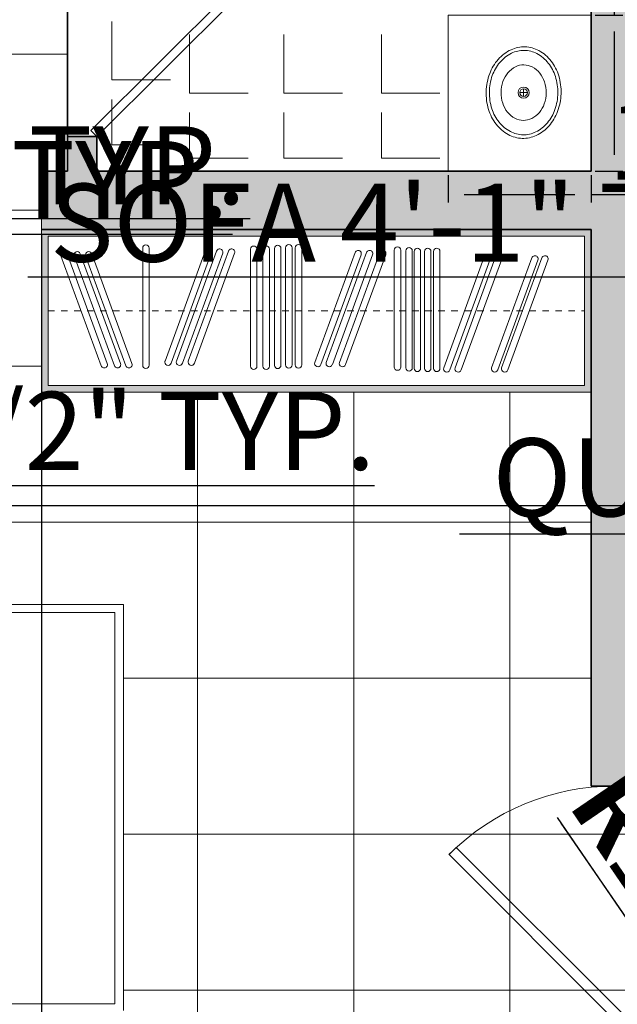
# Model space of a CAD drawing. Units: millimetres. Extents: x 542930 to 543750, y 628093 to 628738.
# Tile 4 of 14: x 543061 to 543153, y 628363 to 628514. Entities that reach past the tile are written whole.
import ezdxf

# ---------------------------------------------------------------- set-up
doc = ezdxf.new("R2010")
doc.units = ezdxf.units.MM
doc.linetypes.add('JIS_02_1.0', pattern=[2, 1, -1])
for name, color, linetype, lineweight in [('A-ANNO-DIMS', 2, 'Continuous', 18), ('A-FLOR-FIXT', 9, 'Continuous', 18), ('A-FURN', 8, 'Continuous', 18), ('A-FURN-MILL', 8, 'Continuous', 18), ('A-FURN-MILL-HIDN', 8, 'JIS_02_1.0', 13), ('A-FURN-PATT', 9, 'Continuous', 13), ('A-WALL', 7, 'Continuous', 35), ('DOORS', 30, 'Continuous', 18)]:
    doc.layers.add(name, color=color, linetype=linetype, lineweight=lineweight)
doc.layers.add('A-FLOR-PATT', color=241, linetype='Continuous', lineweight=13, true_color=0xf7abae)
doc.layers.add('A-WALL-PATT', color=251, linetype='Continuous', lineweight=13, true_color=0x636466)
doc.styles.get("Standard").update_dxf_attribs({"font": 'arial.ttf'})
doc.dimstyles.new('ISO-25', dxfattribs={"dimtxt": 12, "dimasz": 2.5, "dimexe": 1.25, "dimexo": 0.625, "dimtad": 1, "dimdec": 0, "dimlunit": 3, "dimtxsty": 'Standard', "dimcen": 2.5, "dimadec": 0, "dimazin": 0, "dimtfac": 1, "dimtdec": 0, "dimtmove": 0, "dimatfit": 3, "dimfxl": 1, "dimarcsym": 0})

# ---------------------------------------------------------------- blocks, each defined once
blk = doc.blocks.new('*U4')
for p, q in [((0, 0), (0, -6)), ((40, 0), (40, -6))]:
    blk.add_line(p, q)
blk.add_lwpolyline([(0, 0), (28.28, 28.28), (29.52, 27.05), (1.24, -1.24)], close=True)
blk.add_arc((0, 0), 40, 0, 45)
blk = doc.blocks.new('*U3')
for p, q in [((-40, 0), (-40, -6)), ((0, 0), (0, -6))]:
    blk.add_line(p, q)
blk.add_lwpolyline([(0, 0), (-28.28, 28.28), (-29.52, 27.05), (-1.24, -1.24)], close=True)
blk.add_arc((0, 0), 40, 135, 180)
blk = doc.blocks.new('Sink - Oval top')
for p, q in [((-1, 0), (1, 0)), ((0, 1), (0, -1))]:
    blk.add_line(p, q)
for points in [[(-12.23, 0.39, 0.117634), (-11.46, -3.36, 0.104469), (-8.88, -6.8, 0.090016), (-5.08, -9.07, 0.08192), (-0.32, -10.02, 0.08192), (4.49, -9.38, 0.090016), (8.42, -7.36, 0.104469), (11.22, -4.09, 0.117634), (12.23, -0.39, 0.117634), (11.46, 3.36, 0.104469), (8.88, 6.8, 0.090016), (5.08, 9.07, 0.08192), (0.32, 10.02, 0.08192), (-4.49, 9.38, 0.090016), (-8.42, 7.36, 0.104469), (-11.22, 4.09, 0.117634)], [(-11.29, 0.16, 0.118622), (-10.52, -3.25, 0.104678), (-8.07, -6.36, 0.089562), (-4.54, -8.37, 0.081185), (-0.13, -9.15, 0.081185), (4.3, -8.49, 0.089562), (7.89, -6.58, 0.104678), (10.42, -3.55, 0.118622), (11.29, -0.16, 0.118622), (10.52, 3.25, 0.104678), (8.07, 6.36, 0.089562), (4.54, 8.37, 0.081185), (0.13, 9.15, 0.081185), (-4.3, 8.49, 0.089562), (-7.89, 6.58, 0.104678), (-10.42, 3.55, 0.118622)], [(-7.42, 0.08, 0.118283), (-6.91, -2.17, 0.104607), (-5.29, -4.21, 0.089718), (-2.97, -5.53, 0.081436), (-0.07, -6.04, 0.081436), (2.84, -5.59, 0.089718), (5.2, -4.33, 0.104607), (6.86, -2.32, 0.118283), (7.42, -0.08, 0.118283), (6.91, 2.17, 0.104607), (5.29, 4.21, 0.089718), (2.97, 5.53, 0.081436), (0.07, 6.04, 0.081436), (-2.84, 5.59, 0.089718), (-5.2, 4.33, 0.104607), (-6.86, 2.32, 0.118283)]]:
    blk.add_lwpolyline(points, format="xyb", close=True)
for radius in [1.5, 1]:
    blk.add_circle((0, 0), radius)
blk = doc.blocks.new('Bed - Queen')
for p, q in [((0, -80.00003), (0, 0)), ((0, 0), (59.99999, 0)), ((59.99999, 0), (59.99999, -80.00003)), ((7.99999, -1.2), (28.79998, -1.2)), ((7.99999, -14.4), (7.99999, -1.2)), ((28.79998, -1.2), (28.79998, -14.4)), ((31.19999, -1.2), (51.99999, -1.2)), ((31.19999, -14.4), (31.19999, -1.2)), ((51.99999, -1.2), (51.99999, -16.4)), ((0, -14.4), (44.8, -14.4)), ((59.99999, -29.6), (44.8, -14.4)), ((44.8, -14.4), (44.8, -29.6)), ((51.99999, -16.4), (46.79936, -16.4)), ((44.8, -16.8), (0, -16.8)), ((44.8, -29.6), (59.99999, -29.6)), ((59.99999, -80.00003), (0, -80.00003))]:
    blk.add_line(p, q)
blk = doc.blocks.new('WARDROBE-BED-RAIL')
for p, q in [((0, 23), (0, 0)), ((0, 23), (82.5, 23)), ((82.5, 0), (82.5, 23)), ((8.16, 3.05), (1.98, 19.95)), ((9.1, 3.39), (2.92, 20.3)), ((10.2, 3.05), (4.02, 19.95)), ((11.14, 3.39), (4.96, 20.3)), ((11.95, 3.05), (5.77, 19.95)), ((12.89, 3.39), (6.71, 20.3)), ((14.55, 3.16), (14.55, 21.16)), ((15.55, 3.16), (15.55, 21.16)), ((17.99, 3.79), (24.17, 20.7)), ((18.92, 3.45), (25.1, 20.36)), ((19.74, 3.79), (25.92, 20.7)), ((20.68, 3.45), (26.86, 20.36)), ((21.57, 3.79), (27.75, 20.7)), ((22.51, 3.45), (28.69, 20.36)), ((31.12, 2.98), (31.12, 20.98)), ((32.12, 2.98), (32.12, 20.98)), ((33.04, 2.98), (33.04, 20.98)), ((34.04, 2.98), (34.04, 20.98)), ((34.81, 3.12), (34.81, 21.12)), ((35.81, 3.12), (35.81, 21.12)), ((36.51, 3.19), (36.51, 21.19)), ((37.51, 3.19), (37.51, 21.19)), ((38, 3.19), (38, 21.19)), ((39, 3.19), (39, 21.19)), ((41.02, 3.57), (47.2, 20.48)), ((41.96, 3.23), (48.14, 20.14)), ((42.77, 3.57), (48.95, 20.48)), ((43.71, 3.23), (49.89, 20.14)), ((44.81, 3.57), (50.99, 20.48)), ((45.75, 3.23), (51.93, 20.14)), ((53.23, 2.86), (53.23, 20.86)), ((54.23, 2.86), (54.23, 20.86)), ((55, 2.73), (55, 20.73)), ((56, 2.73), (56, 20.73)), ((56.28, 2.66), (56.28, 20.66)), ((57.28, 2.66), (57.28, 20.66)), ((57.87, 2.66), (57.87, 20.66)), ((58.87, 2.66), (58.87, 20.66)), ((59.26, 2.66), (59.26, 20.66)), ((60.26, 2.66), (60.26, 20.66)), ((60.83, 2.75), (67.01, 19.66)), ((61.77, 2.41), (67.95, 19.31)), ((62.58, 2.75), (68.76, 19.66)), ((63.52, 2.41), (69.7, 19.31)), ((68.19, 2.75), (74.37, 19.66)), ((69.13, 2.41), (75.31, 19.31)), ((69.74, 2.75), (75.92, 19.66)), ((70.68, 2.41), (76.86, 19.31)), ((0, 0), (82.5, 0))]:
    blk.add_line(p, q)
for centre, start, end in [((15.05, 21.16), 0, 180), ((31.62, 20.98), 0, 180), ((33.54, 20.98), 0, 180), ((35.31, 21.12), 0, 180), ((37.01, 21.19), 0, 180), ((38.5, 21.19), 0, 180), ((53.73, 20.86), 0, 180), ((55.5, 20.73), 0, 180), ((2.45, 20.12), 20.081, 200.081), ((4.49, 20.12), 20.081, 200.081), ((6.24, 20.12), 20.081, 200.081), ((24.63, 20.53), 339.919, 159.919), ((26.39, 20.53), 339.919, 159.919), ((28.22, 20.53), 339.919, 159.919), ((47.67, 20.31), 339.919, 159.919), ((49.42, 20.31), 339.919, 159.919), ((51.46, 20.31), 339.919, 159.919), ((56.78, 20.66), 0, 180), ((58.37, 20.66), 0, 180), ((59.76, 20.66), 0, 180), ((67.48, 19.49), 339.919, 159.919), ((69.23, 19.49), 339.919, 159.919), ((74.84, 19.49), 339.919, 159.919), ((76.39, 19.49), 339.919, 159.919), ((8.63, 3.22), 200.081, 20.081), ((10.67, 3.22), 200.081, 20.081), ((12.42, 3.22), 200.081, 20.081), ((15.05, 3.16), 180, 0), ((18.45, 3.62), 159.919, 339.919), ((20.21, 3.62), 159.919, 339.919), ((22.04, 3.62), 159.919, 339.919), ((35.31, 3.12), 180, 0), ((37.01, 3.19), 180, 0), ((38.5, 3.19), 180, 0), ((41.49, 3.4), 159.919, 339.919), ((43.24, 3.4), 159.919, 339.919), ((45.28, 3.4), 159.919, 339.919), ((31.62, 2.98), 180, 0), ((33.54, 2.98), 180, 0), ((53.73, 2.86), 180, 0), ((55.5, 2.73), 180, 0), ((56.78, 2.66), 180, 0), ((58.37, 2.66), 180, 0), ((59.76, 2.66), 180, 0), ((61.3, 2.58), 159.919, 339.919), ((63.05, 2.58), 159.919, 339.919), ((68.66, 2.58), 159.919, 339.919), ((70.21, 2.58), 159.919, 339.919)]:
    blk.add_arc(centre, 0.5, start, end)
blk = doc.blocks.new('LAVATORY-COUNTER')
for p, q in [((0, 0), (0, 24)), ((0, 24), (22, 24))]:
    blk.add_line(p, q)
blk = doc.blocks.new('*D32')
at = {"layer": 'A-ANNO-DIMS', "color": 0, "lineweight": -2, "transparency": 16777216}
for p, q in [((543011.12, 628481.15), (543008.62, 628481.15)), ((543013.62, 628478.92), (543013.62, 628482.4)), ((543013.62, 628481.15), (543014.62, 628481.15)), ((543014.62, 628478.92), (543014.62, 628482.4)), ((543017.12, 628481.15), (543094.01, 628481.15))]:
    blk.add_line(p, q, dxfattribs=at)
at = {"layer": 'A-ANNO-DIMS', "color": 0, "transparency": 16777216}
for points in [[(543011.12, 628481.56), (543011.12, 628480.73), (543013.62, 628481.15)], [(543017.12, 628481.56), (543017.12, 628480.73), (543014.62, 628481.15)]]:
    blk.add_solid(points, dxfattribs=at)
at = {"layer": 'Defpoints', "color": 0, "transparency": 16777216}
for p in [(543014.62, 628481.15), (543013.62, 628478.3), (543014.62, 628478.3)]:
    blk.add_point(p, dxfattribs=at)
at = {"layer": 'A-ANNO-DIMS', "color": 0, "transparency": 16777216, "insert": (543056.82, 628487.9), "char_height": 12, "attachment_point": 5}
blk.add_mtext('0\'-1" TYP.', dxfattribs=at)
blk = doc.blocks.new('*D33')
at = {"layer": 'A-ANNO-DIMS', "color": 0, "lineweight": -2, "transparency": 16777216}
for p, q in [((543189.7, 628481.25), (543189.7, 628473.25)), ((543238.84, 628481.25), (543238.84, 628473.25)), ((543189.7, 628474.5), (543062.56, 628474.5)), ((543236.34, 628474.5), (543192.2, 628474.5))]:
    blk.add_line(p, q, dxfattribs=at)
at = {"layer": 'A-ANNO-DIMS', "color": 0, "transparency": 16777216}
for points in [[(543192.2, 628474.92), (543192.2, 628474.09), (543189.7, 628474.5)], [(543236.34, 628474.92), (543236.34, 628474.09), (543238.84, 628474.5)]]:
    blk.add_solid(points, dxfattribs=at)
at = {"layer": 'Defpoints', "color": 0, "transparency": 16777216}
for p in [(543189.7, 628481.87), (543238.84, 628481.87), (543189.7, 628474.5)]:
    blk.add_point(p, dxfattribs=at)
at = {"layer": 'A-ANNO-DIMS', "color": 0, "transparency": 16777216, "insert": (543124.88, 628481.34), "char_height": 12, "attachment_point": 5}
blk.add_mtext('SOFA 4\'-1" TYP.', dxfattribs=at)
blk = doc.blocks.new('*D37')
at = {"layer": 'A-ANNO-DIMS', "color": 0, "lineweight": -2, "transparency": 16777216}
for p, q in [((543337.17, 628423.55), (543337.17, 628436.21)), ((543417.44, 628423.55), (543417.44, 628436.21)), ((543337.17, 628434.96), (543128.93, 628434.96)), ((543414.94, 628434.96), (543339.67, 628434.96))]:
    blk.add_line(p, q, dxfattribs=at)
at = {"layer": 'A-ANNO-DIMS', "color": 0, "transparency": 16777216}
for points in [[(543339.67, 628435.38), (543339.67, 628434.55), (543337.17, 628434.96)], [(543414.94, 628435.38), (543414.94, 628434.55), (543417.44, 628434.96)]]:
    blk.add_solid(points, dxfattribs=at)
at = {"layer": 'Defpoints', "color": 0, "transparency": 16777216}
for p in [(543337.17, 628434.96), (543337.17, 628422.92), (543417.44, 628422.92)]:
    blk.add_point(p, dxfattribs=at)
at = {"layer": 'A-ANNO-DIMS', "color": 0, "transparency": 16777216, "insert": (543231.8, 628442.16), "char_height": 12, "attachment_point": 5}
blk.add_mtext('QUEEN BED 6\'-8 1/2" TYP.', dxfattribs=at)
blk = doc.blocks.new('*D44')
at = {"layer": 'A-ANNO-DIMS', "color": 0, "lineweight": -2, "transparency": 16777216}
for p, q in [((542994.67, 628492.2), (542994.67, 628482.28)), ((543019.67, 628492.2), (543019.67, 628482.28)), ((542997.17, 628483.53), (543017.17, 628483.53)), ((543019.67, 628483.53), (543096.77, 628483.53))]:
    blk.add_line(p, q, dxfattribs=at)
at = {"layer": 'A-ANNO-DIMS', "color": 0, "transparency": 16777216}
for points in [[(542997.17, 628483.94), (542997.17, 628483.11), (542994.67, 628483.53)], [(543017.17, 628483.94), (543017.17, 628483.11), (543019.67, 628483.53)]]:
    blk.add_solid(points, dxfattribs=at)
at = {"layer": 'Defpoints', "color": 0, "transparency": 16777216}
for p in [(542994.67, 628492.83), (543019.67, 628492.83), (543019.67, 628483.53)]:
    blk.add_point(p, dxfattribs=at)
at = {"layer": 'A-ANNO-DIMS', "color": 0, "transparency": 16777216, "insert": (543059.47, 628490.18), "char_height": 12, "attachment_point": 5}
blk.add_mtext('2\'-1" TYP.', dxfattribs=at)
blk = doc.blocks.new('*D55')
at = {"layer": 'A-ANNO-DIMS', "color": 0, "lineweight": -2, "transparency": 16777216}
for p, q in [((543152.77, 628514.83), (543152.77, 628679.13)), ((543149.79, 628514.83), (543154.02, 628514.83)), ((543152.77, 628493.33), (543152.77, 628512.33)), ((543149.79, 628490.83), (543154.02, 628490.83))]:
    blk.add_line(p, q, dxfattribs=at)
at = {"layer": 'A-ANNO-DIMS', "color": 0, "transparency": 16777216}
for points in [[(543152.35, 628512.33), (543153.18, 628512.33), (543152.77, 628514.83)], [(543152.35, 628493.33), (543153.18, 628493.33), (543152.77, 628490.83)]]:
    blk.add_solid(points, dxfattribs=at)
at = {"layer": 'Defpoints', "color": 0, "transparency": 16777216}
for p in [(543149.17, 628514.83), (543152.77, 628514.83), (543149.17, 628490.83)]:
    blk.add_point(p, dxfattribs=at)
at = {"layer": 'A-ANNO-DIMS', "color": 0, "transparency": 16777216, "insert": (543145.93, 628598.23), "char_height": 12, "attachment_point": 5, "rotation": 90}
blk.add_mtext('COUNTER 2\'-0" TYP.', dxfattribs=at)
blk = doc.blocks.new('*D56')
at = {"layer": 'A-ANNO-DIMS', "color": 0, "lineweight": -2, "transparency": 16777216}
for p, q in [((543127.17, 628490.2), (543127.17, 628485.98)), ((543149.17, 628490.2), (543149.17, 628485.98)), ((543129.67, 628487.23), (543146.67, 628487.23)), ((543149.17, 628487.23), (543234.26, 628487.23))]:
    blk.add_line(p, q, dxfattribs=at)
at = {"layer": 'A-ANNO-DIMS', "color": 0, "transparency": 16777216}
for points in [[(543129.67, 628487.64), (543129.67, 628486.81), (543127.17, 628487.23)], [(543146.67, 628487.64), (543146.67, 628486.81), (543149.17, 628487.23)]]:
    blk.add_solid(points, dxfattribs=at)
at = {"layer": 'Defpoints', "color": 0, "transparency": 16777216}
for p in [(543127.17, 628490.83), (543149.17, 628490.83), (543149.17, 628487.23)]:
    blk.add_point(p, dxfattribs=at)
at = {"layer": 'A-ANNO-DIMS', "color": 0, "transparency": 16777216, "insert": (543192.96, 628493.98), "char_height": 12, "attachment_point": 5}
blk.add_mtext('1\'-10" TYP.', dxfattribs=at)
blk = doc.blocks.new('*D60')
at = {"layer": 'A-ANNO-DIMS', "color": 0, "lineweight": -2, "transparency": 16777216}
for p, q in [((542992.67, 628439.52), (542992.67, 628443.74)), ((543012.12, 628439.52), (543012.12, 628443.74)), ((542995.17, 628442.49), (543009.62, 628442.49)), ((543012.12, 628442.49), (543115.85, 628442.49))]:
    blk.add_line(p, q, dxfattribs=at)
at = {"layer": 'A-ANNO-DIMS', "color": 0, "transparency": 16777216}
for points in [[(542995.17, 628442.91), (542995.17, 628442.08), (542992.67, 628442.49)], [(543009.62, 628442.91), (543009.62, 628442.08), (543012.12, 628442.49)]]:
    blk.add_solid(points, dxfattribs=at)
at = {"layer": 'Defpoints', "color": 0, "transparency": 16777216}
for p in [(543012.12, 628442.49), (542992.67, 628438.89), (543012.12, 628438.89)]:
    blk.add_point(p, dxfattribs=at)
at = {"layer": 'A-ANNO-DIMS', "color": 0, "transparency": 16777216, "insert": (543065.24, 628449.32), "char_height": 12, "attachment_point": 5}
blk.add_mtext('1\'-7 1/2" TYP.', dxfattribs=at)
blk = doc.blocks.new('*D75')
at = {"layer": 'A-ANNO-DIMS', "color": 0, "lineweight": -2, "transparency": 16777216}
for p, q in [((543324.54, 628439.36), (542953.72, 628439.36)), ((542954.97, 628352.33), (542954.97, 628436.86)), ((543324.54, 628349.83), (542953.72, 628349.83))]:
    blk.add_line(p, q, dxfattribs=at)
at = {"layer": 'A-ANNO-DIMS', "color": 0, "transparency": 16777216}
for points in [[(542954.55, 628436.86), (542955.38, 628436.86), (542954.97, 628439.36)], [(542954.55, 628352.33), (542955.38, 628352.33), (542954.97, 628349.83)]]:
    blk.add_solid(points, dxfattribs=at)
at = {"layer": 'Defpoints', "color": 0, "transparency": 16777216}
for p in [(542954.97, 628439.36), (543325.17, 628439.36), (543325.17, 628349.83)]:
    blk.add_point(p, dxfattribs=at)
at = {"layer": 'A-ANNO-DIMS', "color": 0, "transparency": 16777216, "insert": (542948.14, 628394.6), "char_height": 12, "attachment_point": 5, "rotation": 90}
blk.add_mtext('7\'-5 1/2"', dxfattribs=at)
blk = doc.blocks.new('*D85')
at = {"layer": 'A-ANNO-DIMS', "color": 0, "lineweight": -2, "transparency": 16777216}
for p, q in [((543028.62, 628481.2), (543028.62, 628103.84)), ((543064.67, 628481.2), (543064.67, 628103.84)), ((543031.12, 628105.09), (543062.17, 628105.09))]:
    blk.add_line(p, q, dxfattribs=at)
at = {"layer": 'A-ANNO-DIMS', "color": 0, "transparency": 16777216}
for points in [[(543031.12, 628105.5), (543031.12, 628104.67), (543028.62, 628105.09)], [(543062.17, 628105.5), (543062.17, 628104.67), (543064.67, 628105.09)]]:
    blk.add_solid(points, dxfattribs=at)
at = {"layer": 'Defpoints', "color": 0, "transparency": 16777216}
for p in [(543028.62, 628481.83), (543064.67, 628481.83), (543064.67, 628105.09)]:
    blk.add_point(p, dxfattribs=at)
at = {"layer": 'A-ANNO-DIMS', "color": 0, "transparency": 16777216, "insert": (543046.65, 628111.84), "char_height": 12, "attachment_point": 5}
blk.add_mtext('3\'-0"', dxfattribs=at)
blk = doc.blocks.new('*D94')
at = {"layer": 'A-ANNO-DIMS', "color": 0, "lineweight": -2, "transparency": 16777216}
for p, q in [((543143.96, 628391.37), (543186.37, 628329.39)), ((543198.34, 628311.9), (543187.78, 628327.33))]:
    blk.add_line(p, q, dxfattribs=at)
at = {"layer": 'A-ANNO-DIMS', "color": 0, "transparency": 16777216}
blk.add_solid([(543186.71, 628329.63), (543186.02, 628329.15), (543187.78, 628327.33)], dxfattribs=at)
at = {"layer": 'Defpoints', "color": 0, "transparency": 16777216}
for p in [(543187.78, 628327.33), (543198.34, 628311.9)]:
    blk.add_point(p, dxfattribs=at)
at = {"layer": 'A-ANNO-DIMS', "color": 0, "transparency": 16777216, "insert": (543170.1, 628365.27), "char_height": 12, "attachment_point": 5, "rotation": 304.3793}
blk.add_mtext('R1\'-6 1/2"', dxfattribs=at)
blk = doc.blocks.new('*D95')
at = {"layer": 'A-ANNO-DIMS', "color": 0, "lineweight": -2, "transparency": 16777216}
for p, q in [((543144.53, 628390.54), (543186.93, 628328.57)), ((543198.34, 628311.9), (543188.34, 628326.5))]:
    blk.add_line(p, q, dxfattribs=at)
at = {"layer": 'A-ANNO-DIMS', "color": 0, "transparency": 16777216}
blk.add_solid([(543187.28, 628328.8), (543186.59, 628328.33), (543188.34, 628326.5)], dxfattribs=at)
at = {"layer": 'Defpoints', "color": 0, "transparency": 16777216}
for p in [(543188.34, 628326.5), (543198.34, 628311.9)]:
    blk.add_point(p, dxfattribs=at)
at = {"layer": 'A-ANNO-DIMS', "color": 0, "transparency": 16777216, "insert": (543170.66, 628364.44), "char_height": 12, "attachment_point": 5, "rotation": 304.3778}
blk.add_mtext('R1\'-5 1/2"', dxfattribs=at)

msp = doc.modelspace()

# ---------------------------------------------------------------- hatches: boundary and pattern name
at = {"layer": 'A-FURN-PATT'}
h = msp.add_hatch(color=256, dxfattribs=at)
h.dxf.hatch_style = 1
h.paths.add_polyline_path([(543149.17, 628481.83), (543064.67, 628481.83), (543064.67, 628456.83), (543149.17, 628456.83)])
h.paths.add_polyline_path([(543065.67, 628480.83), (543148.17, 628480.83), (543148.17, 628457.83), (543065.67, 628457.83)], flags=16)
h.paths.add_polyline_path([(543067.65, 628477.78, -1), (543068.59, 628478.12), (543071.8, 628469.33), (543072.77, 628469.33), (543069.68, 628477.78, -1), (543070.62, 628478.12), (543073.84, 628469.33), (543074.53, 628469.33), (543071.44, 628477.78, -1), (543072.38, 628478.12), (543075.59, 628469.33), (543080.22, 628469.33), (543080.22, 628478.99, -1), (543081.22, 628478.99), (543081.22, 628469.33), (543086.47, 628469.33), (543089.83, 628478.53, -1), (543090.77, 628478.18), (543087.53, 628469.33), (543088.22, 628469.33), (543091.59, 628478.53, -1), (543092.53, 628478.18), (543089.29, 628469.33), (543090.05, 628469.33), (543093.41, 628478.53, -1), (543094.35, 628478.18), (543091.11, 628469.33), (543096.79, 628469.33), (543096.79, 628478.81, -1), (543097.79, 628478.81), (543097.79, 628469.33), (543098.7, 628469.33), (543098.7, 628478.81, -1), (543099.7, 628478.81), (543099.7, 628469.33), (543100.48, 628469.33), (543100.48, 628478.95, -1), (543101.48, 628478.95), (543101.48, 628469.33), (543102.18, 628469.33), (543102.18, 628479.02, -1), (543103.18, 628479.02), (543103.18, 628469.33), (543103.67, 628469.33), (543103.67, 628479.02, -1), (543104.67, 628479.02), (543104.67, 628469.33), (543109.58, 628469.33), (543112.87, 628478.31, -1), (543113.81, 628477.96), (543110.65, 628469.33), (543111.34, 628469.33), (543114.62, 628478.31, -1), (543115.56, 628477.96), (543112.4, 628469.33), (543113.38, 628469.33), (543116.66, 628478.31, -1), (543117.6, 628477.96), (543114.44, 628469.33), (543118.89, 628469.33), (543118.89, 628478.68, -1), (543119.89, 628478.68), (543119.89, 628469.33), (543120.67, 628469.33), (543120.67, 628478.56, -1), (543121.67, 628478.56), (543121.67, 628469.33), (543121.95, 628469.33), (543121.95, 628478.49, -1), (543122.95, 628478.49), (543122.95, 628469.33), (543123.53, 628469.33), (543123.53, 628478.49, -1), (543124.53, 628478.49), (543124.53, 628469.33), (543124.93, 628469.33), (543124.93, 628478.49, -1), (543125.93, 628478.49), (543125.93, 628469.33), (543129.69, 628469.33), (543132.68, 628477.48, -1), (543133.61, 628477.14), (543130.76, 628469.33), (543131.45, 628469.33), (543134.43, 628477.48, -1), (543135.37, 628477.14), (543132.51, 628469.33), (543137.05, 628469.33), (543140.03, 628477.48, -1), (543140.97, 628477.14), (543138.12, 628469.33), (543138.6, 628469.33), (543141.59, 628477.48, -1), (543142.52, 628477.14), (543136.34, 628460.23, -1), (543135.41, 628460.58), (543138.6, 628469.33), (543138.12, 628469.33), (543134.79, 628460.23, -1), (543133.85, 628460.58), (543137.05, 628469.33), (543132.51, 628469.33), (543129.19, 628460.23, -1), (543128.25, 628460.58), (543131.45, 628469.33), (543130.76, 628469.33), (543127.43, 628460.23, -1), (543126.5, 628460.58), (543129.69, 628469.33), (543125.93, 628469.33), (543125.93, 628460.49, -1), (543124.93, 628460.49), (543124.93, 628469.33), (543124.53, 628469.33), (543124.53, 628460.49, -1), (543123.53, 628460.49), (543123.53, 628469.33), (543122.95, 628469.33), (543122.95, 628460.49, -1), (543121.95, 628460.49), (543121.95, 628469.33), (543121.67, 628469.33), (543121.67, 628460.56, -1), (543120.67, 628460.56), (543120.67, 628469.33), (543119.89, 628469.33), (543119.89, 628460.68, -1), (543118.89, 628460.68), (543118.89, 628469.33), (543114.44, 628469.33), (543111.42, 628461.06, -1), (543110.48, 628461.4), (543113.38, 628469.33), (543112.4, 628469.33), (543109.38, 628461.06, -1), (543108.44, 628461.4), (543111.34, 628469.33), (543110.65, 628469.33), (543107.63, 628461.06, -1), (543106.69, 628461.4), (543109.58, 628469.33), (543104.67, 628469.33), (543104.67, 628461.02, -1), (543103.67, 628461.02), (543103.67, 628469.33), (543103.18, 628469.33), (543103.18, 628461.02, -1), (543102.18, 628461.02), (543102.18, 628469.33), (543101.48, 628469.33), (543101.48, 628460.95, -1), (543100.48, 628460.95), (543100.48, 628469.33), (543099.7, 628469.33), (543099.7, 628460.81, -1), (543098.7, 628460.81), (543098.7, 628469.33), (543097.79, 628469.33), (543097.79, 628460.81, -1), (543096.79, 628460.81), (543096.79, 628469.33), (543091.11, 628469.33), (543088.17, 628461.28, -1), (543087.23, 628461.62), (543090.05, 628469.33), (543089.29, 628469.33), (543086.35, 628461.28, -1), (543085.41, 628461.62), (543088.22, 628469.33), (543087.53, 628469.33), (543084.59, 628461.28, -1), (543083.65, 628461.62), (543086.47, 628469.33), (543081.22, 628469.33), (543081.22, 628460.99, -1), (543080.22, 628460.99), (543080.22, 628469.33), (543075.59, 628469.33), (543078.56, 628461.22, -1), (543077.62, 628460.87), (543074.53, 628469.33), (543073.84, 628469.33), (543076.8, 628461.22, -1), (543075.86, 628460.87), (543072.77, 628469.33), (543071.8, 628469.33), (543074.77, 628461.22, -1), (543073.83, 628460.87)], flags=0)
at = {"layer": 'A-WALL-PATT'}
h = msp.add_hatch(color=256, dxfattribs=at)
h.dxf.hatch_style = 1
h.paths.add_polyline_path([(543158.17, 628580.83), (543211.67, 628580.83), (543211.67, 628589.83), (543137.07, 628589.83), (543137.07, 628580.83), (543149.17, 628580.83), (543149.17, 628490.83), (543073.17, 628490.83), (543073.17, 628496.14), (543068.67, 628496.14), (543068.67, 628490.83), (543064.67, 628490.83), (543064.67, 628481.83), (543149.17, 628481.83), (543149.17, 628396.23), (543158.17, 628396.23)])

# ---------------------------------------------------------------- linework, layer by layer
at = {"layer": 'A-FLOR-PATT'}
for p, q in [((543075.49, 628513.86), (543075.49, 628504.86)), ((543087.43, 628511.83), (543087.43, 628502.83)), ((543101.92, 628511.83), (543101.92, 628502.83)), ((543116.93, 628511.83), (543116.93, 628502.83)), ((543021.67, 628508.83), (543068.67, 628508.83)), ((543075.49, 628504.86), (543084.49, 628504.86)), ((543087.43, 628502.83), (543096.43, 628502.83)), ((543101.92, 628502.83), (543110.92, 628502.83)), ((543116.93, 628502.83), (543125.93, 628502.83)), ((543075.49, 628501.86), (543075.49, 628494.86)), ((543087.43, 628499.83), (543087.43, 628492.83)), ((543101.92, 628499.83), (543101.92, 628492.83)), ((543116.93, 628499.83), (543116.93, 628492.83)), ((543075.49, 628494.86), (543084.49, 628494.86)), ((543087.43, 628492.83), (543096.43, 628492.83)), ((543101.92, 628492.83), (543110.92, 628492.83)), ((543116.93, 628492.83), (543125.93, 628492.83)), ((543028.62, 628484.83), (543064.67, 628484.83)), ((543028.62, 628460.83), (543064.67, 628460.83)), ((543088.67, 628262.83), (543088.67, 628456.83)), ((543112.67, 628262.83), (543112.67, 628456.83)), ((543136.67, 628262.83), (543136.67, 628456.83)), ((543012.12, 628436.83), (543149.17, 628436.83)), ((543077.27, 628412.83), (543149.17, 628412.83)), ((543077.27, 628388.83), (543304.67, 628388.83)), ((543077.27, 628364.83), (543304.67, 628364.83))]:
    msp.add_line(p, q, dxfattribs=at)
at = {"layer": 'A-FURN'}
for p, q in [((543012.12, 628424.17), (543077.27, 628424.17)), ((543077.27, 628424.17), (543077.27, 628361.72))]:
    msp.add_line(p, q, dxfattribs=at)
at = {"layer": 'A-FURN-MILL'}
for p, q in [((543064.67, 628490.83), (543064.67, 628456.83)), ((543064.67, 628456.83), (543149.17, 628456.83))]:
    msp.add_line(p, q, dxfattribs=at)
at = {"layer": 'A-FURN-MILL-HIDN'}
msp.add_line((543065.67, 628469.33), (543148.17, 628469.33), dxfattribs=at)
at = {"layer": 'A-WALL'}
for p, q in [((543068.67, 628490.83), (543068.67, 628580.83)), ((543149.17, 628490.83), (543149.17, 628580.83)), ((543068.67, 628496.14), (543073.17, 628496.14)), ((543073.17, 628490.83), (543073.17, 628496.14)), ((543064.67, 628490.83), (543068.67, 628490.83)), ((543073.17, 628490.83), (543149.17, 628490.83)), ((543064.67, 628481.83), (543149.17, 628481.83)), ((543149.17, 628396.23), (543149.17, 628481.83)), ((543158.17, 628396.23), (543149.17, 628396.23))]:
    msp.add_line(p, q, dxfattribs=at)

# ---------------------------------------------------------------- block references
at = {"layer": 'A-FLOR-FIXT'}
msp.add_blockref('LAVATORY-COUNTER', (543127.17, 628490.83), dxfattribs=at)
at = {"layer": 'A-FLOR-FIXT', "xscale": 0.5752271451798996, "yscale": 0.5752271451798996, "zscale": 0.5752271451798996, "rotation": 270}
msp.add_blockref('Sink - Oval top', (543138.79, 628502.91), dxfattribs=at)
at = {"layer": 'A-FURN', "xscale": 1.003451310197957, "yscale": 1.003451310197957, "zscale": 1.003451310197957, "rotation": 90}
msp.add_blockref('Bed - Queen', (542995.67, 628362.72), dxfattribs=at)
at = {"layer": 'A-FURN-MILL'}
msp.add_blockref('WARDROBE-BED-RAIL', (543065.67, 628457.83), dxfattribs=at)
at = {"layer": 'DOORS'}
for name, p, xscale, yscale, zscale, rotation in [('*U3', (543073.17, 628496.14), 0.75, 0.75, 0.75, 270), ('*U4', (543152.77, 628360.23), 0.9000000000029102, 0.9000000000029102, 0.9000000000029102, 90)]:
    msp.add_blockref(name, p, dxfattribs=dict(at, xscale=xscale, yscale=yscale, zscale=zscale, rotation=rotation))

# ---------------------------------------------------------------- dimensions: what is measured, and where the dimension line sits
at = {"layer": 'A-ANNO-DIMS'}
for base, p1, p2, angle, text, picture, middle in [((543152.77, 628514.83), (543149.17, 628490.83), (543149.17, 628514.83), 90, 'COUNTER <> TYP.', '*D55', (543145.93, 628598.23)), ((543189.7, 628474.5), (543238.84, 628481.87), (543189.7, 628481.87), 180, 'SOFA <> TYP.', '*D33', (543124.88, 628481.34)), ((543337.17, 628434.96), (543417.44, 628422.92), (543337.17, 628422.92), 180, 'QUEEN BED <> TYP.', '*D37', (543231.8, 628442.16))]:
    dim = msp.add_linear_dim(base=base, p1=p1, p2=p2, angle=angle, text=text, dimstyle='ISO-25', override={"dimdec": 1, "dimlfac": 1, "dimrnd": 0, "dimzin": 1, "dimdsep": 46, "dimlunit": 4, "dimfrac": 2}, dxfattribs=at)
    dim.commit()
    dim.dimension.update_dxf_attribs({"geometry": picture, "text_midpoint": middle})
for base, p1, p2, picture, middle in [((543149.17, 628487.23), (543127.17, 628490.83), (543149.17, 628490.83), '*D56', (543192.96, 628493.98)), ((543019.67, 628483.53), (542994.67, 628492.83), (543019.67, 628492.83), '*D44', (543059.47, 628490.18)), ((543014.62, 628481.15), (543013.62, 628478.3), (543014.62, 628478.3), '*D32', (543056.82, 628487.9)), ((543012.1235, 628442.4945), (542992.6669, 628438.8945), (543012.1235, 628438.8945), '*D60', (543065.2376, 628449.3241))]:
    dim = msp.add_linear_dim(base=base, p1=p1, p2=p2, text='<> TYP.', dimstyle='ISO-25', override={"dimdec": 1, "dimlfac": 1, "dimrnd": 0, "dimzin": 1, "dimdsep": 46, "dimlunit": 4, "dimfrac": 2}, dxfattribs=at)
    dim.commit()
    dim.dimension.update_dxf_attribs({"geometry": picture, "text_midpoint": middle})
dim = msp.add_linear_dim(base=(543064.6669, 628105.0858), p1=(543028.6237, 628481.8258), p2=(543064.6669, 628481.8258), dimstyle='ISO-25', override={"dimdec": 1, "dimlfac": 1, "dimrnd": 0, "dimzin": 1, "dimdsep": 46, "dimlunit": 4, "dimfrac": 2}, dxfattribs=at)
dim.commit()
dim.dimension.update_dxf_attribs({"geometry": '*D85', "text_midpoint": (543046.6453, 628111.8418)})
dim = msp.add_linear_dim(base=(542954.97, 628439.36), p1=(543325.17, 628349.83), p2=(543325.17, 628439.36), angle=90, dimstyle='ISO-25', override={"dimdec": 1, "dimlfac": 1, "dimrnd": 0, "dimzin": 1, "dimdsep": 46, "dimlunit": 4, "dimfrac": 2}, dxfattribs=at)
dim.commit()
dim.dimension.update_dxf_attribs({"geometry": '*D75', "text_midpoint": (542948.14, 628394.6)})
for mpoint, picture, middle in [((543187.78, 628327.33), '*D94', (543170.1, 628365.27)), ((543188.34, 628326.5), '*D95', (543170.66, 628364.44))]:
    dim = msp.add_radius_dim(center=(543198.34, 628311.9), mpoint=mpoint, dimstyle='ISO-25', override={"dimdec": 1, "dimlfac": 1, "dimrnd": 0, "dimzin": 1, "dimdsep": 46, "dimlunit": 4, "dimfrac": 2}, dxfattribs=at)
    dim.commit()
    dim.dimension.update_dxf_attribs({"geometry": picture, "text_midpoint": middle})

doc.saveas('drawing.dxf')
